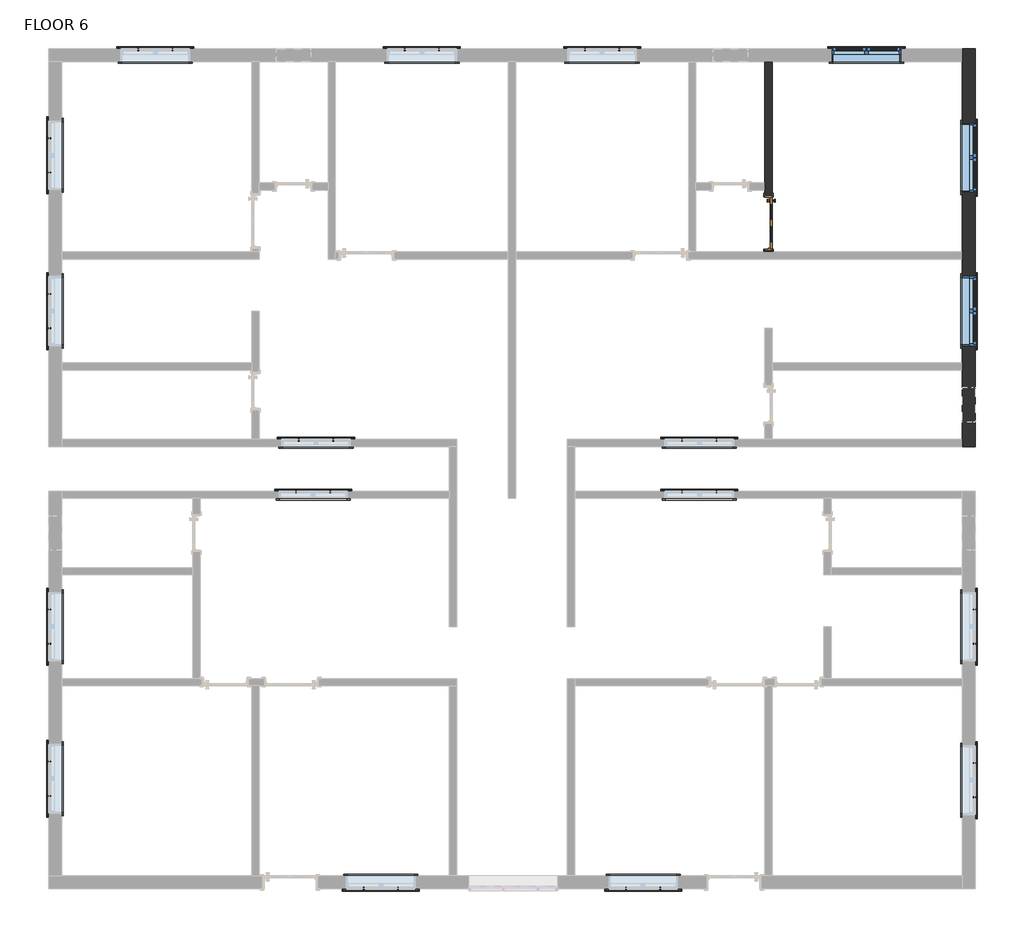
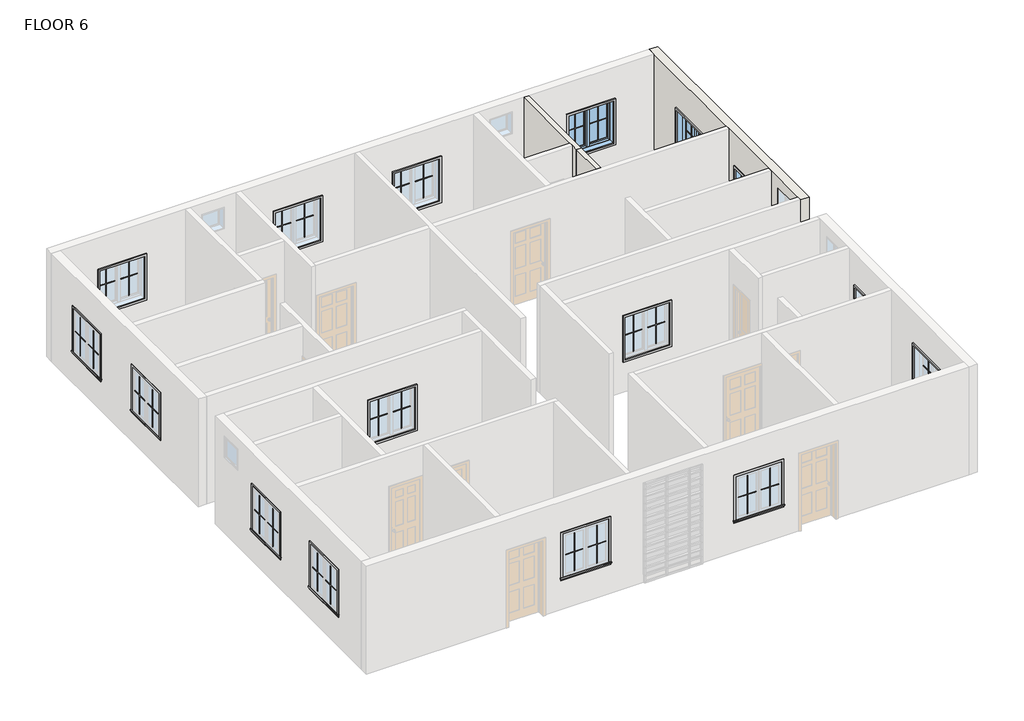
# One storey, part 4 of 4: 72 proxies, 3 walls, 3 windows, 1 door.
"""IFC4 building model written with IfcOpenShell, lengths in millimetres."""

from ifc_helpers import new_model, si_unit, frame, origin, place, context, project, spatial, polyline, outline, extrude, faceted_brep, transform, mapped, element, save
from components import muntin_pattern_2x2_muntin_pattern_2x2_4dfeb3f3, muntin_pattern_2x2_muntin_pattern_2x2_e852a7e4, trim_window_exterior_flat_with_sill_7cfdd449, trim_window_interior_flat_picture_frame_f1e0b15b, door_03e3dfb5, window_9200f5ac

model = new_model("IFC4")

# Units and contexts
model_context = context("Model", 3, world=origin())
ifc_project = project(units=[si_unit("LENGTHUNIT", "METRE", prefix="MILLI")], contexts=[model_context])

# Site, building, storey
site = spatial("IfcSite", under=ifc_project)
building = spatial("IfcBuilding", under=site)
storey = spatial("IfcBuildingStorey", under=building, Name="FLOOR 6", Elevation=9544.3725604)

# Proxies
placement = place(None, origin())
muntin_pattern_2x2_muntin_pattern_2x2_shape = muntin_pattern_2x2_muntin_pattern_2x2_4dfeb3f3(model_context)
element("IfcBuildingElementProxy", 1, Name="Muntin Pattern_2x2 : Muntin Pattern_2x2", ObjectType="Muntin Pattern_2x2 : Muntin Pattern_2x2", at=placement, inside=storey, context=model_context, shape_type="MappedRepresentation", body=[
    mapped(muntin_pattern_2x2_muntin_pattern_2x2_shape, transform((-12420.8887331, 2059.7281164, 10528.6225604), x_axis=(0.0, 1.0, 0.0), y_axis=(-1.0, 0.0, 0.0), z_axis=(0.0, 0.0, 1.0))),
])
element("IfcBuildingElementProxy", 2, Name="Muntin Pattern_2x2 : Muntin Pattern_2x2", ObjectType="Muntin Pattern_2x2 : Muntin Pattern_2x2", at=placement, inside=storey, context=model_context, shape_type="MappedRepresentation", body=[
    mapped(muntin_pattern_2x2_muntin_pattern_2x2_shape, transform((-12420.8887331, 4803.7218664, 10528.6225604), x_axis=(0.0, 1.0, 0.0), y_axis=(-1.0, 0.0, 0.0), z_axis=(0.0, 0.0, 1.0))),
])
element("IfcBuildingElementProxy", 3, Name="Muntin Pattern_2x2 : Muntin Pattern_2x2", ObjectType="Muntin Pattern_2x2 : Muntin Pattern_2x2", at=placement, inside=storey, context=model_context, shape_type="MappedRepresentation", body=[
    mapped(muntin_pattern_2x2_muntin_pattern_2x2_shape, transform((-10854.0262331, 6977.8031164, 10528.6225604), x_axis=(1.0, 0.0, 0.0), y_axis=(0.0, 1.0, 0.0), z_axis=(0.0, 0.0, 1.0))),
])
element("IfcBuildingElementProxy", 4, Name="Muntin Pattern_2x2 : Muntin Pattern_2x2", ObjectType="Muntin Pattern_2x2 : Muntin Pattern_2x2", at=placement, inside=storey, context=model_context, shape_type="MappedRepresentation", body=[
    mapped(muntin_pattern_2x2_muntin_pattern_2x2_shape, transform((-6155.0262331, 6977.8031164, 10528.6225604), x_axis=(1.0, 0.0, 0.0), y_axis=(0.0, 1.0, 0.0), z_axis=(0.0, 0.0, 1.0))),
])
element("IfcBuildingElementProxy", 5, Name="Muntin Pattern_2x2 : Muntin Pattern_2x2", ObjectType="Muntin Pattern_2x2 : Muntin Pattern_2x2", at=placement, inside=storey, context=model_context, shape_type="MappedRepresentation", body=[
    mapped(muntin_pattern_2x2_muntin_pattern_2x2_shape, transform((-2980.0262331, 6977.8031164, 10528.6225604), x_axis=(1.0, 0.0, 0.0), y_axis=(0.0, 1.0, 0.0), z_axis=(0.0, 0.0, 1.0))),
])
element("IfcBuildingElementProxy", 6, Name="Muntin Pattern_2x2 : Muntin Pattern_2x2", ObjectType="Muntin Pattern_2x2 : Muntin Pattern_2x2", at=placement, inside=storey, context=model_context, shape_type="MappedRepresentation", body=[
    mapped(muntin_pattern_2x2_muntin_pattern_2x2_shape, transform((1680.8737669, 6977.8031164, 10528.6225604), x_axis=(1.0, 0.0, 0.0), y_axis=(0.0, 1.0, 0.0), z_axis=(0.0, 0.0, 1.0))),
])
element("IfcBuildingElementProxy", 7, Name="Muntin Pattern_2x2 : Muntin Pattern_2x2", ObjectType="Muntin Pattern_2x2 : Muntin Pattern_2x2", at=placement, inside=storey, context=model_context, shape_type="MappedRepresentation", body=[
    mapped(muntin_pattern_2x2_muntin_pattern_2x2_shape, transform((3892.2612669, 5371.2531164, 10528.6225604), x_axis=(0.0, -1.0, 0.0), y_axis=(1.0, 0.0, 0.0), z_axis=(0.0, 0.0, 1.0))),
])
element("IfcBuildingElementProxy", 8, Name="Muntin Pattern_2x2 : Muntin Pattern_2x2", ObjectType="Muntin Pattern_2x2 : Muntin Pattern_2x2", at=placement, inside=storey, context=model_context, shape_type="MappedRepresentation", body=[
    mapped(muntin_pattern_2x2_muntin_pattern_2x2_shape, transform((3892.2612669, 2666.1531164, 10528.6225604), x_axis=(0.0, -1.0, 0.0), y_axis=(1.0, 0.0, 0.0), z_axis=(0.0, 0.0, 1.0))),
])
element("IfcBuildingElementProxy", 9, Name="Muntin Pattern_2x2 : Muntin Pattern_2x2", ObjectType="Muntin Pattern_2x2 : Muntin Pattern_2x2", at=placement, inside=storey, context=model_context, shape_type="MappedRepresentation", body=[
    mapped(muntin_pattern_2x2_muntin_pattern_2x2_shape, transform((3892.2612669, -2896.4468836, 10528.6225604), x_axis=(0.0, -1.0, 0.0), y_axis=(1.0, 0.0, 0.0), z_axis=(0.0, 0.0, 1.0))),
])
element("IfcBuildingElementProxy", 10, Name="Muntin Pattern_2x2 : Muntin Pattern_2x2", ObjectType="Muntin Pattern_2x2 : Muntin Pattern_2x2", at=placement, inside=storey, context=model_context, shape_type="MappedRepresentation", body=[
    mapped(muntin_pattern_2x2_muntin_pattern_2x2_shape, transform((3892.2612669, -5601.5468836, 10528.6225604), x_axis=(0.0, -1.0, 0.0), y_axis=(1.0, 0.0, 0.0), z_axis=(0.0, 0.0, 1.0))),
])
element("IfcBuildingElementProxy", 11, Name="Muntin Pattern_2x2 : Muntin Pattern_2x2", ObjectType="Muntin Pattern_2x2 : Muntin Pattern_2x2", at=placement, inside=storey, context=model_context, shape_type="MappedRepresentation", body=[
    mapped(muntin_pattern_2x2_muntin_pattern_2x2_shape, transform((-1649.7012331, -7812.9343836, 10528.6225604), x_axis=(-1.0, 0.0, 0.0), y_axis=(0.0, -1.0, 0.0), z_axis=(0.0, 0.0, 1.0))),
])
element("IfcBuildingElementProxy", 12, Name="Muntin Pattern_2x2 : Muntin Pattern_2x2", ObjectType="Muntin Pattern_2x2 : Muntin Pattern_2x2", at=placement, inside=storey, context=model_context, shape_type="MappedRepresentation", body=[
    mapped(muntin_pattern_2x2_muntin_pattern_2x2_shape, transform((-6272.5012331, -7812.9343836, 10528.6225604), x_axis=(-1.0, 0.0, 0.0), y_axis=(0.0, -1.0, 0.0), z_axis=(0.0, 0.0, 1.0))),
])
element("IfcBuildingElementProxy", 13, Name="Muntin Pattern_2x2 : Muntin Pattern_2x2", ObjectType="Muntin Pattern_2x2 : Muntin Pattern_2x2", at=placement, inside=storey, context=model_context, shape_type="MappedRepresentation", body=[
    mapped(muntin_pattern_2x2_muntin_pattern_2x2_shape, transform((-12420.8887331, -6182.5718836, 10528.6225604), x_axis=(0.0, 1.0, 0.0), y_axis=(-1.0, 0.0, 0.0), z_axis=(0.0, 0.0, 1.0))),
])
element("IfcBuildingElementProxy", 14, Name="Muntin Pattern_2x2 : Muntin Pattern_2x2", ObjectType="Muntin Pattern_2x2 : Muntin Pattern_2x2", at=placement, inside=storey, context=model_context, shape_type="MappedRepresentation", body=[
    mapped(muntin_pattern_2x2_muntin_pattern_2x2_shape, transform((-12420.8887331, -3502.8718836, 10528.6225604), x_axis=(0.0, 1.0, 0.0), y_axis=(-1.0, 0.0, 0.0), z_axis=(0.0, 0.0, 1.0))),
])
element("IfcBuildingElementProxy", 15, Name="Muntin Pattern_2x2 : Muntin Pattern_2x2", ObjectType="Muntin Pattern_2x2 : Muntin Pattern_2x2", at=placement, inside=storey, context=model_context, shape_type="MappedRepresentation", body=[
    mapped(muntin_pattern_2x2_muntin_pattern_2x2_shape, transform((-8072.7262331, -821.5843836, 10528.6225604), x_axis=(1.0, 0.0, 0.0), y_axis=(0.0, 1.0, 0.0), z_axis=(0.0, 0.0, 1.0))),
])
element("IfcBuildingElementProxy", 16, Name="Muntin Pattern_2x2 : Muntin Pattern_2x2", ObjectType="Muntin Pattern_2x2 : Muntin Pattern_2x2", at=placement, inside=storey, context=model_context, shape_type="MappedRepresentation", body=[
    mapped(muntin_pattern_2x2_muntin_pattern_2x2_shape, transform((-8021.9262331, 92.8156164, 10528.6225604), x_axis=(1.0, 0.0, 0.0), y_axis=(0.0, 1.0, 0.0), z_axis=(0.0, 0.0, 1.0))),
])
element("IfcBuildingElementProxy", 17, Name="Muntin Pattern_2x2 : Muntin Pattern_2x2", ObjectType="Muntin Pattern_2x2 : Muntin Pattern_2x2", at=placement, inside=storey, context=model_context, shape_type="MappedRepresentation", body=[
    mapped(muntin_pattern_2x2_muntin_pattern_2x2_shape, transform((-1265.5262331, -821.5843836, 10528.6225604), x_axis=(1.0, 0.0, 0.0), y_axis=(0.0, 1.0, 0.0), z_axis=(0.0, 0.0, 1.0))),
])
element("IfcBuildingElementProxy", 18, Name="Muntin Pattern_2x2 : Muntin Pattern_2x2", ObjectType="Muntin Pattern_2x2 : Muntin Pattern_2x2", at=placement, inside=storey, context=model_context, shape_type="MappedRepresentation", body=[
    mapped(muntin_pattern_2x2_muntin_pattern_2x2_shape, transform((-1265.5262331, 92.8156164, 10528.6225604), x_axis=(1.0, 0.0, 0.0), y_axis=(0.0, 1.0, 0.0), z_axis=(0.0, 0.0, 1.0))),
])
muntin_pattern_2x2_muntin_pattern_2x2_2_shape = muntin_pattern_2x2_muntin_pattern_2x2_e852a7e4(model_context)
element("IfcBuildingElementProxy", 19, Name="Muntin Pattern_2x2 : Muntin Pattern_2x2", ObjectType="Muntin Pattern_2x2 : Muntin Pattern_2x2", at=placement, inside=storey, context=model_context, shape_type="MappedRepresentation", body=[
    mapped(muntin_pattern_2x2_muntin_pattern_2x2_2_shape, transform((-12420.8887331, 2666.1531164, 10528.6225604), x_axis=(0.0, -1.0, 0.0), y_axis=(1.0, 0.0, 0.0), z_axis=(0.0, 0.0, 1.0))),
])
element("IfcBuildingElementProxy", 20, Name="Muntin Pattern_2x2 : Muntin Pattern_2x2", ObjectType="Muntin Pattern_2x2 : Muntin Pattern_2x2", at=placement, inside=storey, context=model_context, shape_type="MappedRepresentation", body=[
    mapped(muntin_pattern_2x2_muntin_pattern_2x2_2_shape, transform((-12420.8887331, 5410.1468664, 10528.6225604), x_axis=(0.0, -1.0, 0.0), y_axis=(1.0, 0.0, 0.0), z_axis=(0.0, 0.0, 1.0))),
])
element("IfcBuildingElementProxy", 21, Name="Muntin Pattern_2x2 : Muntin Pattern_2x2", ObjectType="Muntin Pattern_2x2 : Muntin Pattern_2x2", at=placement, inside=storey, context=model_context, shape_type="MappedRepresentation", body=[
    mapped(muntin_pattern_2x2_muntin_pattern_2x2_2_shape, transform((-10247.6012331, 6977.8031164, 10528.6225604), x_axis=(-1.0, 0.0, 0.0), y_axis=(0.0, -1.0, 0.0), z_axis=(0.0, 0.0, 1.0))),
])
element("IfcBuildingElementProxy", 22, Name="Muntin Pattern_2x2 : Muntin Pattern_2x2", ObjectType="Muntin Pattern_2x2 : Muntin Pattern_2x2", at=placement, inside=storey, context=model_context, shape_type="MappedRepresentation", body=[
    mapped(muntin_pattern_2x2_muntin_pattern_2x2_2_shape, transform((-5548.6012331, 6977.8031164, 10528.6225604), x_axis=(-1.0, 0.0, 0.0), y_axis=(0.0, -1.0, 0.0), z_axis=(0.0, 0.0, 1.0))),
])
element("IfcBuildingElementProxy", 23, Name="Muntin Pattern_2x2 : Muntin Pattern_2x2", ObjectType="Muntin Pattern_2x2 : Muntin Pattern_2x2", at=placement, inside=storey, context=model_context, shape_type="MappedRepresentation", body=[
    mapped(muntin_pattern_2x2_muntin_pattern_2x2_2_shape, transform((-2373.6012331, 6977.8031164, 10528.6225604), x_axis=(-1.0, 0.0, 0.0), y_axis=(0.0, -1.0, 0.0), z_axis=(0.0, 0.0, 1.0))),
])
element("IfcBuildingElementProxy", 24, Name="Muntin Pattern_2x2 : Muntin Pattern_2x2", ObjectType="Muntin Pattern_2x2 : Muntin Pattern_2x2", at=placement, inside=storey, context=model_context, shape_type="MappedRepresentation", body=[
    mapped(muntin_pattern_2x2_muntin_pattern_2x2_2_shape, transform((2287.2987669, 6977.8031164, 10528.6225604), x_axis=(-1.0, 0.0, 0.0), y_axis=(0.0, -1.0, 0.0), z_axis=(0.0, 0.0, 1.0))),
])
element("IfcBuildingElementProxy", 25, Name="Muntin Pattern_2x2 : Muntin Pattern_2x2", ObjectType="Muntin Pattern_2x2 : Muntin Pattern_2x2", at=placement, inside=storey, context=model_context, shape_type="MappedRepresentation", body=[
    mapped(muntin_pattern_2x2_muntin_pattern_2x2_2_shape, transform((3892.2612669, 4764.8281164, 10528.6225604), x_axis=(0.0, 1.0, 0.0), y_axis=(-1.0, 0.0, 0.0), z_axis=(0.0, 0.0, 1.0))),
])
element("IfcBuildingElementProxy", 26, Name="Muntin Pattern_2x2 : Muntin Pattern_2x2", ObjectType="Muntin Pattern_2x2 : Muntin Pattern_2x2", at=placement, inside=storey, context=model_context, shape_type="MappedRepresentation", body=[
    mapped(muntin_pattern_2x2_muntin_pattern_2x2_2_shape, transform((3892.2612669, 2059.7281164, 10528.6225604), x_axis=(0.0, 1.0, 0.0), y_axis=(-1.0, 0.0, 0.0), z_axis=(0.0, 0.0, 1.0))),
])
element("IfcBuildingElementProxy", 27, Name="Muntin Pattern_2x2 : Muntin Pattern_2x2", ObjectType="Muntin Pattern_2x2 : Muntin Pattern_2x2", at=placement, inside=storey, context=model_context, shape_type="MappedRepresentation", body=[
    mapped(muntin_pattern_2x2_muntin_pattern_2x2_2_shape, transform((3892.2612669, -3502.8718836, 10528.6225604), x_axis=(0.0, 1.0, 0.0), y_axis=(-1.0, 0.0, 0.0), z_axis=(0.0, 0.0, 1.0))),
])
element("IfcBuildingElementProxy", 28, Name="Muntin Pattern_2x2 : Muntin Pattern_2x2", ObjectType="Muntin Pattern_2x2 : Muntin Pattern_2x2", at=placement, inside=storey, context=model_context, shape_type="MappedRepresentation", body=[
    mapped(muntin_pattern_2x2_muntin_pattern_2x2_2_shape, transform((3892.2612669, -6207.9718836, 10528.6225604), x_axis=(0.0, 1.0, 0.0), y_axis=(-1.0, 0.0, 0.0), z_axis=(0.0, 0.0, 1.0))),
])
element("IfcBuildingElementProxy", 29, Name="Muntin Pattern_2x2 : Muntin Pattern_2x2", ObjectType="Muntin Pattern_2x2 : Muntin Pattern_2x2", at=placement, inside=storey, context=model_context, shape_type="MappedRepresentation", body=[
    mapped(muntin_pattern_2x2_muntin_pattern_2x2_2_shape, transform((-2256.1262331, -7812.9343836, 10528.6225604), x_axis=(1.0, 0.0, 0.0), y_axis=(0.0, 1.0, 0.0), z_axis=(0.0, 0.0, 1.0))),
])
element("IfcBuildingElementProxy", 30, Name="Muntin Pattern_2x2 : Muntin Pattern_2x2", ObjectType="Muntin Pattern_2x2 : Muntin Pattern_2x2", at=placement, inside=storey, context=model_context, shape_type="MappedRepresentation", body=[
    mapped(muntin_pattern_2x2_muntin_pattern_2x2_2_shape, transform((-6878.9262331, -7812.9343836, 10528.6225604), x_axis=(1.0, 0.0, 0.0), y_axis=(0.0, 1.0, 0.0), z_axis=(0.0, 0.0, 1.0))),
])
element("IfcBuildingElementProxy", 31, Name="Muntin Pattern_2x2 : Muntin Pattern_2x2", ObjectType="Muntin Pattern_2x2 : Muntin Pattern_2x2", at=placement, inside=storey, context=model_context, shape_type="MappedRepresentation", body=[
    mapped(muntin_pattern_2x2_muntin_pattern_2x2_2_shape, transform((-12420.8887331, -5576.1468836, 10528.6225604), x_axis=(0.0, -1.0, 0.0), y_axis=(1.0, 0.0, 0.0), z_axis=(0.0, 0.0, 1.0))),
])
element("IfcBuildingElementProxy", 32, Name="Muntin Pattern_2x2 : Muntin Pattern_2x2", ObjectType="Muntin Pattern_2x2 : Muntin Pattern_2x2", at=placement, inside=storey, context=model_context, shape_type="MappedRepresentation", body=[
    mapped(muntin_pattern_2x2_muntin_pattern_2x2_2_shape, transform((-12420.8887331, -2896.4468836, 10528.6225604), x_axis=(0.0, -1.0, 0.0), y_axis=(1.0, 0.0, 0.0), z_axis=(0.0, 0.0, 1.0))),
])
element("IfcBuildingElementProxy", 33, Name="Muntin Pattern_2x2 : Muntin Pattern_2x2", ObjectType="Muntin Pattern_2x2 : Muntin Pattern_2x2", at=placement, inside=storey, context=model_context, shape_type="MappedRepresentation", body=[
    mapped(muntin_pattern_2x2_muntin_pattern_2x2_2_shape, transform((-7466.3012331, -821.5843836, 10528.6225604), x_axis=(-1.0, 0.0, 0.0), y_axis=(0.0, -1.0, 0.0), z_axis=(0.0, 0.0, 1.0))),
])
element("IfcBuildingElementProxy", 34, Name="Muntin Pattern_2x2 : Muntin Pattern_2x2", ObjectType="Muntin Pattern_2x2 : Muntin Pattern_2x2", at=placement, inside=storey, context=model_context, shape_type="MappedRepresentation", body=[
    mapped(muntin_pattern_2x2_muntin_pattern_2x2_2_shape, transform((-7415.5012331, 92.8156164, 10528.6225604), x_axis=(-1.0, 0.0, 0.0), y_axis=(0.0, -1.0, 0.0), z_axis=(0.0, 0.0, 1.0))),
])
element("IfcBuildingElementProxy", 35, Name="Muntin Pattern_2x2 : Muntin Pattern_2x2", ObjectType="Muntin Pattern_2x2 : Muntin Pattern_2x2", at=placement, inside=storey, context=model_context, shape_type="MappedRepresentation", body=[
    mapped(muntin_pattern_2x2_muntin_pattern_2x2_2_shape, transform((-659.1012331, -821.5843836, 10528.6225604), x_axis=(-1.0, 0.0, 0.0), y_axis=(0.0, -1.0, 0.0), z_axis=(0.0, 0.0, 1.0))),
])
element("IfcBuildingElementProxy", 36, Name="Muntin Pattern_2x2 : Muntin Pattern_2x2", ObjectType="Muntin Pattern_2x2 : Muntin Pattern_2x2", at=placement, inside=storey, context=model_context, shape_type="MappedRepresentation", body=[
    mapped(muntin_pattern_2x2_muntin_pattern_2x2_2_shape, transform((-659.1012331, 92.8156164, 10528.6225604), x_axis=(-1.0, 0.0, 0.0), y_axis=(0.0, -1.0, 0.0), z_axis=(0.0, 0.0, 1.0))),
])
trim_window_exterior_flat_with_sill_shape = trim_window_exterior_flat_with_sill_7cfdd449(model_context)
element("IfcBuildingElementProxy", 37, Name="Trim-Window-Exterior-Flat : with Sill", ObjectType="Trim-Window-Exterior-Flat : with Sill", at=placement, inside=storey, context=model_context, shape_type="MappedRepresentation", body=[
    mapped(trim_window_exterior_flat_with_sill_shape, transform((-12430.4137331, 2362.9406164, 11677.9725604), x_axis=(0.0, -1.0, 0.0), y_axis=(0.0, 0.0, 1.0), z_axis=(-1.0, 0.0, 0.0))),
])
element("IfcBuildingElementProxy", 38, Name="Trim-Window-Exterior-Flat : with Sill", ObjectType="Trim-Window-Exterior-Flat : with Sill", at=placement, inside=storey, context=model_context, shape_type="MappedRepresentation", body=[
    mapped(trim_window_exterior_flat_with_sill_shape, transform((-12430.4137331, 5106.9343664, 11677.9725604), x_axis=(0.0, -1.0, 0.0), y_axis=(0.0, 0.0, 1.0), z_axis=(-1.0, 0.0, 0.0))),
])
element("IfcBuildingElementProxy", 39, Name="Trim-Window-Exterior-Flat : with Sill", ObjectType="Trim-Window-Exterior-Flat : with Sill", at=placement, inside=storey, context=model_context, shape_type="MappedRepresentation", body=[
    mapped(trim_window_exterior_flat_with_sill_shape, transform((-10550.8137331, 6987.3281164, 11677.9725604), x_axis=(-1.0, 0.0, 0.0), y_axis=(0.0, 0.0, 1.0), z_axis=(0.0, 1.0, 0.0))),
])
element("IfcBuildingElementProxy", 40, Name="Trim-Window-Exterior-Flat : with Sill", ObjectType="Trim-Window-Exterior-Flat : with Sill", at=placement, inside=storey, context=model_context, shape_type="MappedRepresentation", body=[
    mapped(trim_window_exterior_flat_with_sill_shape, transform((-5851.8137331, 6987.3281164, 11677.9725604), x_axis=(-1.0, 0.0, 0.0), y_axis=(0.0, 0.0, 1.0), z_axis=(0.0, 1.0, 0.0))),
])
element("IfcBuildingElementProxy", 41, Name="Trim-Window-Exterior-Flat : with Sill", ObjectType="Trim-Window-Exterior-Flat : with Sill", at=placement, inside=storey, context=model_context, shape_type="MappedRepresentation", body=[
    mapped(trim_window_exterior_flat_with_sill_shape, transform((-2676.8137331, 6987.3281164, 11677.9725604), x_axis=(-1.0, 0.0, 0.0), y_axis=(0.0, 0.0, 1.0), z_axis=(0.0, 1.0, 0.0))),
])
element("IfcBuildingElementProxy", 42, Name="Trim-Window-Exterior-Flat : with Sill", ObjectType="Trim-Window-Exterior-Flat : with Sill", at=placement, inside=storey, context=model_context, shape_type="MappedRepresentation", body=[
    mapped(trim_window_exterior_flat_with_sill_shape, transform((1984.0862669, 6987.3281164, 11677.9725604), x_axis=(-1.0, 0.0, 0.0), y_axis=(0.0, 0.0, 1.0), z_axis=(0.0, 1.0, 0.0))),
])
element("IfcBuildingElementProxy", 43, Name="Trim-Window-Exterior-Flat : with Sill", ObjectType="Trim-Window-Exterior-Flat : with Sill", at=placement, inside=storey, context=model_context, shape_type="MappedRepresentation", body=[
    mapped(trim_window_exterior_flat_with_sill_shape, transform((3901.7862669, 5068.0406164, 11677.9725604), x_axis=(0.0, 1.0, 0.0), y_axis=(0.0, 0.0, 1.0), z_axis=(1.0, 0.0, 0.0))),
])
element("IfcBuildingElementProxy", 44, Name="Trim-Window-Exterior-Flat : with Sill", ObjectType="Trim-Window-Exterior-Flat : with Sill", at=placement, inside=storey, context=model_context, shape_type="MappedRepresentation", body=[
    mapped(trim_window_exterior_flat_with_sill_shape, transform((3901.7862669, 2362.9406164, 11677.9725604), x_axis=(0.0, 1.0, 0.0), y_axis=(0.0, 0.0, 1.0), z_axis=(1.0, 0.0, 0.0))),
])
element("IfcBuildingElementProxy", 45, Name="Trim-Window-Exterior-Flat : with Sill", ObjectType="Trim-Window-Exterior-Flat : with Sill", at=placement, inside=storey, context=model_context, shape_type="MappedRepresentation", body=[
    mapped(trim_window_exterior_flat_with_sill_shape, transform((3901.7862669, -3199.6593836, 11677.9725604), x_axis=(0.0, 1.0, 0.0), y_axis=(0.0, 0.0, 1.0), z_axis=(1.0, 0.0, 0.0))),
])
element("IfcBuildingElementProxy", 46, Name="Trim-Window-Exterior-Flat : with Sill", ObjectType="Trim-Window-Exterior-Flat : with Sill", at=placement, inside=storey, context=model_context, shape_type="MappedRepresentation", body=[
    mapped(trim_window_exterior_flat_with_sill_shape, transform((3901.7862669, -5904.7593836, 11677.9725604), x_axis=(0.0, 1.0, 0.0), y_axis=(0.0, 0.0, 1.0), z_axis=(1.0, 0.0, 0.0))),
])
element("IfcBuildingElementProxy", 47, Name="Trim-Window-Exterior-Flat : with Sill", ObjectType="Trim-Window-Exterior-Flat : with Sill", at=placement, inside=storey, context=model_context, shape_type="MappedRepresentation", body=[
    mapped(trim_window_exterior_flat_with_sill_shape, transform((-1952.9137331, -7822.4593836, 11677.9725604), x_axis=(1.0, 0.0, 0.0), y_axis=(0.0, 0.0, 1.0), z_axis=(0.0, -1.0, 0.0))),
])
element("IfcBuildingElementProxy", 48, Name="Trim-Window-Exterior-Flat : with Sill", ObjectType="Trim-Window-Exterior-Flat : with Sill", at=placement, inside=storey, context=model_context, shape_type="MappedRepresentation", body=[
    mapped(trim_window_exterior_flat_with_sill_shape, transform((-6575.7137331, -7822.4593836, 11677.9725604), x_axis=(1.0, 0.0, 0.0), y_axis=(0.0, 0.0, 1.0), z_axis=(0.0, -1.0, 0.0))),
])
element("IfcBuildingElementProxy", 49, Name="Trim-Window-Exterior-Flat : with Sill", ObjectType="Trim-Window-Exterior-Flat : with Sill", at=placement, inside=storey, context=model_context, shape_type="MappedRepresentation", body=[
    mapped(trim_window_exterior_flat_with_sill_shape, transform((-12430.4137331, -5879.3593836, 11677.9725604), x_axis=(0.0, -1.0, 0.0), y_axis=(0.0, 0.0, 1.0), z_axis=(-1.0, 0.0, 0.0))),
])
element("IfcBuildingElementProxy", 50, Name="Trim-Window-Exterior-Flat : with Sill", ObjectType="Trim-Window-Exterior-Flat : with Sill", at=placement, inside=storey, context=model_context, shape_type="MappedRepresentation", body=[
    mapped(trim_window_exterior_flat_with_sill_shape, transform((-12430.4137331, -3199.6593836, 11677.9725604), x_axis=(0.0, -1.0, 0.0), y_axis=(0.0, 0.0, 1.0), z_axis=(-1.0, 0.0, 0.0))),
])
element("IfcBuildingElementProxy", 51, Name="Trim-Window-Exterior-Flat : with Sill", ObjectType="Trim-Window-Exterior-Flat : with Sill", at=placement, inside=storey, context=model_context, shape_type="MappedRepresentation", body=[
    mapped(trim_window_exterior_flat_with_sill_shape, transform((-7769.5137331, -812.0593836, 11677.9725604), x_axis=(-1.0, 0.0, 0.0), y_axis=(0.0, 0.0, 1.0), z_axis=(0.0, 1.0, 0.0))),
])
element("IfcBuildingElementProxy", 52, Name="Trim-Window-Exterior-Flat : with Sill", ObjectType="Trim-Window-Exterior-Flat : with Sill", at=placement, inside=storey, context=model_context, shape_type="MappedRepresentation", body=[
    mapped(trim_window_exterior_flat_with_sill_shape, transform((-7718.7137331, 102.3406164, 11677.9725604), x_axis=(-1.0, 0.0, 0.0), y_axis=(0.0, 0.0, 1.0), z_axis=(0.0, 1.0, 0.0))),
])
element("IfcBuildingElementProxy", 53, Name="Trim-Window-Exterior-Flat : with Sill", ObjectType="Trim-Window-Exterior-Flat : with Sill", at=placement, inside=storey, context=model_context, shape_type="MappedRepresentation", body=[
    mapped(trim_window_exterior_flat_with_sill_shape, transform((-962.3137331, -812.0593836, 11677.9725604), x_axis=(-1.0, 0.0, 0.0), y_axis=(0.0, 0.0, 1.0), z_axis=(0.0, 1.0, 0.0))),
])
element("IfcBuildingElementProxy", 54, Name="Trim-Window-Exterior-Flat : with Sill", ObjectType="Trim-Window-Exterior-Flat : with Sill", at=placement, inside=storey, context=model_context, shape_type="MappedRepresentation", body=[
    mapped(trim_window_exterior_flat_with_sill_shape, transform((-962.3137331, 102.3406164, 11677.9725604), x_axis=(-1.0, 0.0, 0.0), y_axis=(0.0, 0.0, 1.0), z_axis=(0.0, 1.0, 0.0))),
])
trim_window_interior_flat_picture_frame_shape = trim_window_interior_flat_picture_frame_f1e0b15b(model_context)
element("IfcBuildingElementProxy", 55, Name="Trim-Window-Interior-Flat : Picture Frame", ObjectType="Trim-Window-Interior-Flat : Picture Frame", at=placement, inside=storey, context=model_context, shape_type="MappedRepresentation", body=[
    mapped(trim_window_interior_flat_picture_frame_shape, transform((-12201.8137331, 2362.9406164, 11677.9725604), x_axis=(0.0, 1.0, 0.0), y_axis=(0.0, 0.0, 1.0), z_axis=(1.0, 0.0, 0.0))),
])
element("IfcBuildingElementProxy", 56, Name="Trim-Window-Interior-Flat : Picture Frame", ObjectType="Trim-Window-Interior-Flat : Picture Frame", at=placement, inside=storey, context=model_context, shape_type="MappedRepresentation", body=[
    mapped(trim_window_interior_flat_picture_frame_shape, transform((-12201.8137331, 5106.9343664, 11677.9725604), x_axis=(0.0, 1.0, 0.0), y_axis=(0.0, 0.0, 1.0), z_axis=(1.0, 0.0, 0.0))),
])
element("IfcBuildingElementProxy", 57, Name="Trim-Window-Interior-Flat : Picture Frame", ObjectType="Trim-Window-Interior-Flat : Picture Frame", at=placement, inside=storey, context=model_context, shape_type="MappedRepresentation", body=[
    mapped(trim_window_interior_flat_picture_frame_shape, transform((-10550.8137331, 6758.7281164, 11677.9725604), x_axis=(1.0, 0.0, 0.0), y_axis=(0.0, 0.0, 1.0), z_axis=(0.0, -1.0, 0.0))),
])
element("IfcBuildingElementProxy", 58, Name="Trim-Window-Interior-Flat : Picture Frame", ObjectType="Trim-Window-Interior-Flat : Picture Frame", at=placement, inside=storey, context=model_context, shape_type="MappedRepresentation", body=[
    mapped(trim_window_interior_flat_picture_frame_shape, transform((-5851.8137331, 6758.7281164, 11677.9725604), x_axis=(1.0, 0.0, 0.0), y_axis=(0.0, 0.0, 1.0), z_axis=(0.0, -1.0, 0.0))),
])
element("IfcBuildingElementProxy", 59, Name="Trim-Window-Interior-Flat : Picture Frame", ObjectType="Trim-Window-Interior-Flat : Picture Frame", at=placement, inside=storey, context=model_context, shape_type="MappedRepresentation", body=[
    mapped(trim_window_interior_flat_picture_frame_shape, transform((-2676.8137331, 6758.7281164, 11677.9725604), x_axis=(1.0, 0.0, 0.0), y_axis=(0.0, 0.0, 1.0), z_axis=(0.0, -1.0, 0.0))),
])
element("IfcBuildingElementProxy", 60, Name="Trim-Window-Interior-Flat : Picture Frame", ObjectType="Trim-Window-Interior-Flat : Picture Frame", at=placement, inside=storey, context=model_context, shape_type="MappedRepresentation", body=[
    mapped(trim_window_interior_flat_picture_frame_shape, transform((1984.0862669, 6758.7281164, 11677.9725604), x_axis=(1.0, 0.0, 0.0), y_axis=(0.0, 0.0, 1.0), z_axis=(0.0, -1.0, 0.0))),
])
element("IfcBuildingElementProxy", 61, Name="Trim-Window-Interior-Flat : Picture Frame", ObjectType="Trim-Window-Interior-Flat : Picture Frame", at=placement, inside=storey, context=model_context, shape_type="MappedRepresentation", body=[
    mapped(trim_window_interior_flat_picture_frame_shape, transform((3673.1862669, 5068.0406164, 11677.9725604), x_axis=(0.0, -1.0, 0.0), y_axis=(0.0, 0.0, 1.0), z_axis=(-1.0, 0.0, 0.0))),
])
element("IfcBuildingElementProxy", 62, Name="Trim-Window-Interior-Flat : Picture Frame", ObjectType="Trim-Window-Interior-Flat : Picture Frame", at=placement, inside=storey, context=model_context, shape_type="MappedRepresentation", body=[
    mapped(trim_window_interior_flat_picture_frame_shape, transform((3673.1862669, 2362.9406164, 11677.9725604), x_axis=(0.0, -1.0, 0.0), y_axis=(0.0, 0.0, 1.0), z_axis=(-1.0, 0.0, 0.0))),
])
element("IfcBuildingElementProxy", 63, Name="Trim-Window-Interior-Flat : Picture Frame", ObjectType="Trim-Window-Interior-Flat : Picture Frame", at=placement, inside=storey, context=model_context, shape_type="MappedRepresentation", body=[
    mapped(trim_window_interior_flat_picture_frame_shape, transform((3673.1862669, -3199.6593836, 11677.9725604), x_axis=(0.0, -1.0, 0.0), y_axis=(0.0, 0.0, 1.0), z_axis=(-1.0, 0.0, 0.0))),
])
element("IfcBuildingElementProxy", 64, Name="Trim-Window-Interior-Flat : Picture Frame", ObjectType="Trim-Window-Interior-Flat : Picture Frame", at=placement, inside=storey, context=model_context, shape_type="MappedRepresentation", body=[
    mapped(trim_window_interior_flat_picture_frame_shape, transform((3673.1862669, -5904.7593836, 11677.9725604), x_axis=(0.0, -1.0, 0.0), y_axis=(0.0, 0.0, 1.0), z_axis=(-1.0, 0.0, 0.0))),
])
element("IfcBuildingElementProxy", 65, Name="Trim-Window-Interior-Flat : Picture Frame", ObjectType="Trim-Window-Interior-Flat : Picture Frame", at=placement, inside=storey, context=model_context, shape_type="MappedRepresentation", body=[
    mapped(trim_window_interior_flat_picture_frame_shape, transform((-1952.9137331, -7593.8593836, 11677.9725604), x_axis=(-1.0, 0.0, 0.0), y_axis=(0.0, 0.0, 1.0), z_axis=(0.0, 1.0, 0.0))),
])
element("IfcBuildingElementProxy", 66, Name="Trim-Window-Interior-Flat : Picture Frame", ObjectType="Trim-Window-Interior-Flat : Picture Frame", at=placement, inside=storey, context=model_context, shape_type="MappedRepresentation", body=[
    mapped(trim_window_interior_flat_picture_frame_shape, transform((-6575.7137331, -7593.8593836, 11677.9725604), x_axis=(-1.0, 0.0, 0.0), y_axis=(0.0, 0.0, 1.0), z_axis=(0.0, 1.0, 0.0))),
])
element("IfcBuildingElementProxy", 67, Name="Trim-Window-Interior-Flat : Picture Frame", ObjectType="Trim-Window-Interior-Flat : Picture Frame", at=placement, inside=storey, context=model_context, shape_type="MappedRepresentation", body=[
    mapped(trim_window_interior_flat_picture_frame_shape, transform((-12201.8137331, -5879.3593836, 11677.9725604), x_axis=(0.0, 1.0, 0.0), y_axis=(0.0, 0.0, 1.0), z_axis=(1.0, 0.0, 0.0))),
])
element("IfcBuildingElementProxy", 68, Name="Trim-Window-Interior-Flat : Picture Frame", ObjectType="Trim-Window-Interior-Flat : Picture Frame", at=placement, inside=storey, context=model_context, shape_type="MappedRepresentation", body=[
    mapped(trim_window_interior_flat_picture_frame_shape, transform((-12201.8137331, -3199.6593836, 11677.9725604), x_axis=(0.0, 1.0, 0.0), y_axis=(0.0, 0.0, 1.0), z_axis=(1.0, 0.0, 0.0))),
])
element("IfcBuildingElementProxy", 69, Name="Trim-Window-Interior-Flat : Picture Frame", ObjectType="Trim-Window-Interior-Flat : Picture Frame", at=placement, inside=storey, context=model_context, shape_type="MappedRepresentation", body=[
    mapped(trim_window_interior_flat_picture_frame_shape, transform((-7769.5137331, -939.0593836, 11677.9725604), x_axis=(1.0, 0.0, 0.0), y_axis=(0.0, 0.0, 1.0), z_axis=(0.0, -1.0, 0.0))),
])
element("IfcBuildingElementProxy", 70, Name="Trim-Window-Interior-Flat : Picture Frame", ObjectType="Trim-Window-Interior-Flat : Picture Frame", at=placement, inside=storey, context=model_context, shape_type="MappedRepresentation", body=[
    mapped(trim_window_interior_flat_picture_frame_shape, transform((-7718.7137331, -24.6593836, 11677.9725604), x_axis=(1.0, 0.0, 0.0), y_axis=(0.0, 0.0, 1.0), z_axis=(0.0, -1.0, 0.0))),
])
element("IfcBuildingElementProxy", 71, Name="Trim-Window-Interior-Flat : Picture Frame", ObjectType="Trim-Window-Interior-Flat : Picture Frame", at=placement, inside=storey, context=model_context, shape_type="MappedRepresentation", body=[
    mapped(trim_window_interior_flat_picture_frame_shape, transform((-962.3137331, -939.0593836, 11677.9725604), x_axis=(1.0, 0.0, 0.0), y_axis=(0.0, 0.0, 1.0), z_axis=(0.0, -1.0, 0.0))),
])
element("IfcBuildingElementProxy", 72, Name="Trim-Window-Interior-Flat : Picture Frame", ObjectType="Trim-Window-Interior-Flat : Picture Frame", at=placement, inside=storey, context=model_context, shape_type="MappedRepresentation", body=[
    mapped(trim_window_interior_flat_picture_frame_shape, transform((-962.3137331, -24.6593836, 11677.9725604), x_axis=(1.0, 0.0, 0.0), y_axis=(0.0, 0.0, 1.0), z_axis=(0.0, -1.0, 0.0))),
])

# Door
door_shape = door_03e3dfb5(model_context)
element("IfcDoor", 73, ObjectType="Door-Interior-Single-6_Panel-Wood : 36\" x 84\"", at=placement, inside=storey, context=model_context, shape_type="MappedRepresentation", body=[
    mapped(door_shape, transform((260.0612669, 3912.3406164, 9544.3725604), x_axis=(0.0, -1.0, 0.0), y_axis=(1.0, 0.0, 0.0), z_axis=(0.0, 0.0, 1.0))),
])

# Walls
element("IfcWall", 74, ObjectType="Inner Wall 5\"", at=placement, inside=storey, context=model_context, shape_type="Brep", body=[
    faceted_brep([(320.3862669, 6758.7281164, 12592.3725604), (320.3862669, 4318.7406164, 12592.3725604), (320.3862669, 4318.7406164, 11703.3725604), (320.3862669, 4394.9406164, 11703.3725604), (320.3862669, 4394.9406164, 9544.3725604), (320.3862669, 6758.7281164, 9544.3725604), (193.3862669, 4318.7406164, 12592.3725604), (193.3862669, 4496.5406164, 12592.3725604), (193.3862669, 4623.5406164, 12592.3725604), (193.3862669, 6758.7281164, 12592.3725604), (193.3862669, 6758.7281164, 9544.3725604), (193.3862669, 4623.5406164, 9544.3725604), (193.3862669, 4496.5406164, 9544.3725604), (193.3862669, 4394.9406164, 9544.3725604), (193.3862669, 4394.9406164, 11703.3725604), (193.3862669, 4318.7406164, 11703.3725604)], [[[0, 1, 2, 3, 4, 5]], [[6, 7, 8, 9, 10, 11, 12, 13, 14, 15]], [[10, 5, 4, 13, 12, 11]], [[1, 0, 9, 8, 7, 6]], [[1, 6, 15, 2]], [[0, 5, 10, 9]], [[14, 3, 2, 15]], [[3, 14, 13, 4]]]),
])
element("IfcWall", 75, ObjectType="Inner Wall 5\"", at=placement, inside=storey, context=model_context, shape_type="SweptSolid", body=[
    extrude(outline(polyline([(3404.3406164, 12592.3725604), (4318.7406164, 12592.3725604), (4318.7406164, 11703.3725604), (3429.7406164, 11703.3725604), (3429.7406164, 9544.3725604), (3404.3406164, 9544.3725604), (3404.3406164, 12592.3725604)])), frame((193.3862669, 0.0, 0.0), z_axis=(1.0, 0.0, 0.0), x_axis=(0.0, 1.0, 0.0)), (0.0, 0.0, 1.0), 127.0),
])
element("IfcWall", 76, ObjectType="outer wall 9\"", at=placement, inside=storey, context=model_context, shape_type="Brep", body=[
    faceted_brep([(3673.1862669, 6987.3281164, 9544.3725604), (3673.1862669, 6758.7281164, 9544.3725604), (3673.1862669, 3404.3406164, 9544.3725604), (3673.1862669, 3277.3406164, 9544.3725604), (3673.1862669, 1448.5406164, 9544.3725604), (3673.1862669, 1321.5406164, 9544.3725604), (3673.1862669, 102.3406164, 9544.3725604), (3673.1862669, -24.6593836, 9544.3725604), (3673.1862669, -24.6593836, 12592.3725604), (3673.1862669, 102.3406164, 12592.3725604), (3673.1862669, 1321.5406164, 12592.3725604), (3673.1862669, 1448.5406164, 12592.3725604), (3673.1862669, 3277.3406164, 12592.3725604), (3673.1862669, 3404.3406164, 12592.3725604), (3673.1862669, 6758.7281164, 12592.3725604), (3673.1862669, 6987.3281164, 12592.3725604), (3673.1862669, 4458.4406164, 11677.9725604), (3673.1862669, 4458.4406164, 10458.7725604), (3673.1862669, 5677.6406164, 10458.7725604), (3673.1862669, 5677.6406164, 11677.9725604), (3673.1862669, 1753.3406164, 11677.9725604), (3673.1862669, 1753.3406164, 10458.7725604), (3673.1862669, 2972.5406164, 10458.7725604), (3673.1862669, 2972.5406164, 11677.9725604), (3673.1862669, 407.1406164, 12287.5725604), (3673.1862669, 407.1406164, 11677.9725604), (3673.1862669, 1016.7406164, 11677.9725604), (3673.1862669, 1016.7406164, 12287.5725604), (3901.7862669, 6987.3281164, 9544.3725604), (3901.7862669, 6987.3281164, 12592.3725604), (3901.7862669, -24.6593836, 12592.3725604), (3901.7862669, -24.6593836, 9544.3725604), (3901.7862669, 4458.4406164, 11677.9725604), (3901.7862669, 5677.6406164, 11677.9725604), (3901.7862669, 5677.6406164, 10458.7725604), (3901.7862669, 4458.4406164, 10458.7725604), (3901.7862669, 1753.3406164, 11677.9725604), (3901.7862669, 2972.5406164, 11677.9725604), (3901.7862669, 2972.5406164, 10458.7725604), (3901.7862669, 1753.3406164, 10458.7725604), (3901.7862669, 407.1406164, 12287.5725604), (3901.7862669, 1016.7406164, 12287.5725604), (3901.7862669, 1016.7406164, 11677.9725604), (3901.7862669, 407.1406164, 11677.9725604)], [[[0, 1, 2, 3, 4, 5, 6, 7, 8, 9, 10, 11, 12, 13, 14, 15], [16, 17, 18, 19], [20, 21, 22, 23], [24, 25, 26, 27]], [[28, 29, 30, 31], [32, 33, 34, 35], [36, 37, 38, 39], [40, 41, 42, 43]], [[7, 6, 5, 4, 3, 2, 1, 0, 28, 31]], [[15, 14, 13, 12, 11, 10, 9, 8, 30, 29]], [[0, 15, 29, 28]], [[8, 7, 31, 30]], [[17, 16, 32, 35]], [[18, 17, 35, 34]], [[19, 18, 34, 33]], [[16, 19, 33, 32]], [[21, 20, 36, 39]], [[22, 21, 39, 38]], [[23, 22, 38, 37]], [[20, 23, 37, 36]], [[25, 24, 40, 43]], [[26, 25, 43, 42]], [[27, 26, 42, 41]], [[24, 27, 41, 40]]]),
])

# Windows
window_shape = window_9200f5ac(model_context)
element("IfcWindow", 77, ObjectType="Window-Casement-Double : 48\" x 48\"", at=placement, inside=storey, context=model_context, shape_type="MappedRepresentation", body=[
    mapped(window_shape, transform((1984.0862669, 6873.0281164, 9544.3725604), x_axis=(1.0, 0.0, 0.0), y_axis=(0.0, 1.0, 0.0), z_axis=(0.0, 0.0, 1.0))),
])
element("IfcWindow", 78, ObjectType="Window-Casement-Double : 48\" x 48\"", at=placement, inside=storey, context=model_context, shape_type="MappedRepresentation", body=[
    mapped(window_shape, transform((3787.4862669, 5068.0406164, 9544.3725604), x_axis=(0.0, -1.0, 0.0), y_axis=(1.0, 0.0, 0.0), z_axis=(0.0, 0.0, 1.0))),
])
element("IfcWindow", 79, ObjectType="Window-Casement-Double : 48\" x 48\"", at=placement, inside=storey, context=model_context, shape_type="MappedRepresentation", body=[
    mapped(window_shape, transform((3787.4862669, 2362.9406164, 9544.3725604), x_axis=(0.0, -1.0, 0.0), y_axis=(1.0, 0.0, 0.0), z_axis=(0.0, 0.0, 1.0))),
])

save(model, "model.ifc")

# Revit data of these elements
# Type "Muntin Pattern_2x2 : Muntin Pattern_2x2"
#   Width [instance default] = 4' - 0"
#   Thickness = 0' - 0 1/2"
#   Height [instance default] = 4' - 0"
#   Distance = 0' - 0 3/4"
#   Interior Material [instance default] = none
#   Exterior Material [instance default] = none
#   Default Elevation = 0
# Type "Trim-Window-Exterior-Flat : with Sill"
#   Trim Width = 0' - 2 1/4"
#   Trim Thickness_Picture Frame = 0' - 1 1/4"
#   Trim Thickness_with Sill = 0' - 0 3/4"
#   Sill Thickness = 0' - 1 1/4"
#   Opening Width [instance default] = 2' - 0"
#   Opening Height [instance default] = 3' - 0"
#   Default Elevation = 4' - 0"
#   Sill = yes
#   Picture Frame = no
#   Trim Material [instance default] = none
# Type "Trim-Window-Interior-Flat : Picture Frame"
#   Trim Thickness_Picture Frame = 0' - 1 1/4"
#   Trim Width = 0' - 2 1/4"
#   Trim Thickness_with Sill = 0' - 0 3/4"
#   Sill Thickness = 0' - 1 1/4"
#   Opening Width [instance default] = 2' - 0"
#   Opening Height [instance default] = 3' - 0"
#   Default Elevation = 4' - 0"
#   Sill = no
#   Picture Frame = yes
#   Trim Material [instance default] = none
# Type "Door-Interior-Single-6_Panel-Wood : 36\" x 84\""
#   Type Mark = "8"
#   Assembly Code = "C1020300"
#   Analytic Construction = "Wooden"
#   Top Rail = 0' - 4 11/16"
#   Top Panel = 0' - 11"
#   Thickness = 0' - 1 3/8"
#   Thermal Resistance (R) = 2.5876 (h·ft²·°F)/BTU
#   Swing Angle [instance default] = 90.00°
#   Stiles = 0' - 4 3/4"
#   Rough Width = 3' - 2"
#   Rough Height = 7' - 1"
#   Mullion = 0' - 4 1/2"
#   Lock Rail = 0' - 7 1/2"
#   Intermediate Rail = 0' - 4 1/2"
#   Height = 7' - 0"
#   Width = 3' - 0"
#   Heat Transfer Coefficient (U) = 0.3865 BTU/(h·ft²·°F)
#   Bottom Rail = 0' - 9 1/8"
#   Trim Material = Cherry
#   Panel Material = Cherry
#   Frame Material = Cherry
#   Door Handle Material = Aluminum
#   Visual Light Transmittance = 0
#   Solar Heat Gain Coefficient = 0
#   Wall Closure = (empty or 0)
#   Function = (empty or 0)
# Type "Inner Wall 5\""
#   Assembly Code = "B2010"
#   Layers, outside or top first: 0' - 5" "wall paint" (function 1)
# Type "outer wall 9\""
#   Assembly Code = "B2010"
#   Layers, outside or top first: 0' - 9" "wall paint" (function 1)
# Type "Window-Casement-Double : 48\" x 48\""
#   Type Mark = "18"
#   Fire Rating = "0.5h"
#   Assembly Code = "B2020100"
#   Analytic Construction = "Double glazing - domestic"
#   Frame Extension [instance default] = 0' - 0 1/4"
#   Window Inset [instance default] = 0' - 0"
#   Wall Thickness [instance default] = 0' - 6"
#   Interior Wall Closure [instance default] = 0' - 2 1/4"
#   Half Width = 2' - 0"
#   Visual Light Transmittance = 0.81
#   Thermal Resistance (R) = 1.8146 (h·ft²·°F)/BTU
#   Solar Heat Gain Coefficient = 0.76
#   Rough Width = 4' - 0 1/2"
#   Rough Height = 4' - 0 1/2"
#   Height = 4' - 0"
#   Heat Transfer Coefficient (U) = 0.5511 BTU/(h·ft²·°F)
#   Exterior Wall Closure [instance default] = 0' - 1 1/4"
#   Extension Jamb [instance default] = 0' - 2 1/4"
#   Default Sill Height = 3' - 0"
#   Width = 4' - 0"
#   Muntin Visibility = yes
#   Interior Trim Visibility [instance default] = yes
#   Exterior Trim Visibility [instance default] = yes
#   Extension Jamb Visibility [instance default] = yes
#   Interior Trim Material = Wood - Stained
#   Muntin Pattern = Muntin Pattern_2x2 : Muntin Pattern_2x2
#   Interior Trim = Trim-Window-Interior-Flat : Picture Frame
#   Interior Frame Material = Wood - Stained
#   Glass Panel Material = Glass
#   Exterior Trim Material = Clad - White
#   Exterior Trim = Trim-Window-Exterior-Flat : with Sill
#   Exterior Frame Material = Clad - White
#   Wall Closure = (empty or 0)
# Elements 1, 2, 3, 4, 5, 6, 7, 8, 9, 10, 11, 12, 13, 14, 15, 16, 17, 18, 19, 20, 21, 22, 23, 24, 25, 26, 27, 28, 29, 30, 31, 32, 33, 34, 35, 36 (IfcBuildingElementProxy, "Muntin Pattern_2x2 : Muntin Pattern_2x2")
#   Width = 1' - 6 5/8"
#   Height = 3' - 6 1/2"
#   Interior Material = Wood - Stained
#   Exterior Material = Clad - White
#   Phase Created = New Construction
#   Materials on its faces: "Clad - White", "Wood - Stained"
# Elements 37, 38, 39, 40, 41, 42, 43, 44, 45, 46, 47, 48, 49, 50, 51, 52, 53, 54 (IfcBuildingElementProxy, "Trim-Window-Exterior-Flat : with Sill")
#   Opening Width = 4' - 0"
#   Opening Height = 4' - 0"
#   Trim Material = Clad - White
#   Phase Created = New Construction
#   Materials on its faces: "Clad - White"
# Elements 55, 56, 57, 58, 59, 60, 61, 62, 63, 64, 65, 66, 67, 68, 69, 70, 71, 72 (IfcBuildingElementProxy, "Trim-Window-Interior-Flat : Picture Frame")
#   Opening Width = 4' - 0"
#   Opening Height = 4' - 0"
#   Trim Material = Wood - Stained
#   Phase Created = New Construction
#   Materials on its faces: "Wood - Stained"
# Element 73 (IfcDoor, "Door-Interior-Single-6_Panel-Wood : 36\" x 84\"")
#   Swing Angle = 90.00°
#   Phase Created = New Construction
#   Materials on its faces: "Cherry", "Aluminum"
# Elements 74, 75 (IfcWall, "Inner Wall 5\"")
#   Top Offset = 0' - 0"
#   Base Offset = 0' - 0"
#   Unconnected Height = 10' - 0"
#   wall height = 10' - 0"
#   Phase Created = New Construction
#   Base Constraint = FLOOR 6
#   Materials on its faces: "wall paint"
# Element 76 (IfcWall, "outer wall 9\"")
#   Top Offset = 0' - 0"
#   Base Offset = 0' - 0"
#   Unconnected Height = 10' - 0"
#   wall height = 10' - 0"
#   Phase Created = New Construction
#   Base Constraint = FLOOR 6
#   Materials on its faces: "wall paint", "Clad - White"
# Element 77 (IfcWindow, "Window-Casement-Double : 48\" x 48\"")
#   Mark = "144"
#   Window Inset = 0' - 0"
#   Interior Wall Closure = 0' - 2 1/4"
#   Frame Extension = 0' - 0 1/4"
#   Exterior Wall Closure = 0' - 1 1/4"
#   Interior Trim Visibility = yes
#   Exterior Trim Visibility = yes
#   Phase Created = New Construction
#   Materials on its faces: "Wood - Stained", "Glass", "Clad - White"
# Element 78 (IfcWindow, "Window-Casement-Double : 48\" x 48\"")
#   Mark = "145"
#   Window Inset = 0' - 0"
#   Interior Wall Closure = 0' - 2 1/4"
#   Frame Extension = 0' - 0 1/4"
#   Exterior Wall Closure = 0' - 1 1/4"
#   Interior Trim Visibility = yes
#   Exterior Trim Visibility = yes
#   Phase Created = New Construction
#   Materials on its faces: "Wood - Stained", "Glass", "Clad - White"
# Element 79 (IfcWindow, "Window-Casement-Double : 48\" x 48\"")
#   Mark = "146"
#   Window Inset = 0' - 0"
#   Interior Wall Closure = 0' - 2 1/4"
#   Frame Extension = 0' - 0 1/4"
#   Exterior Wall Closure = 0' - 1 1/4"
#   Interior Trim Visibility = yes
#   Exterior Trim Visibility = yes
#   Phase Created = New Construction
#   Materials on its faces: "Wood - Stained", "Glass", "Clad - White"
# Materials
#   "Cherry": class "Wood", colour RGB 226 177 128, transparency 0, Description = "Prunus Serotina", Cost = 0
#   "Aluminum": class "Metal", colour RGB 247 247 247, transparency 0, Description = "Aluminum 6061", Cost = 0
#   "wall paint": class "Generic", colour RGB 120 120 120, transparency 0, Cost = 0
#   "Wood - Stained": class "Wood", colour RGB 224 178 126, transparency 0, Cost = 0
#   "Glass": class "Glass", colour RGB 0 128 192, transparency 0.75, Description = "Soda Lime Glass", Cost = 0
#   "Clad - White": class "Wood", colour RGB 242 242 238, transparency 0, Cost = 0
